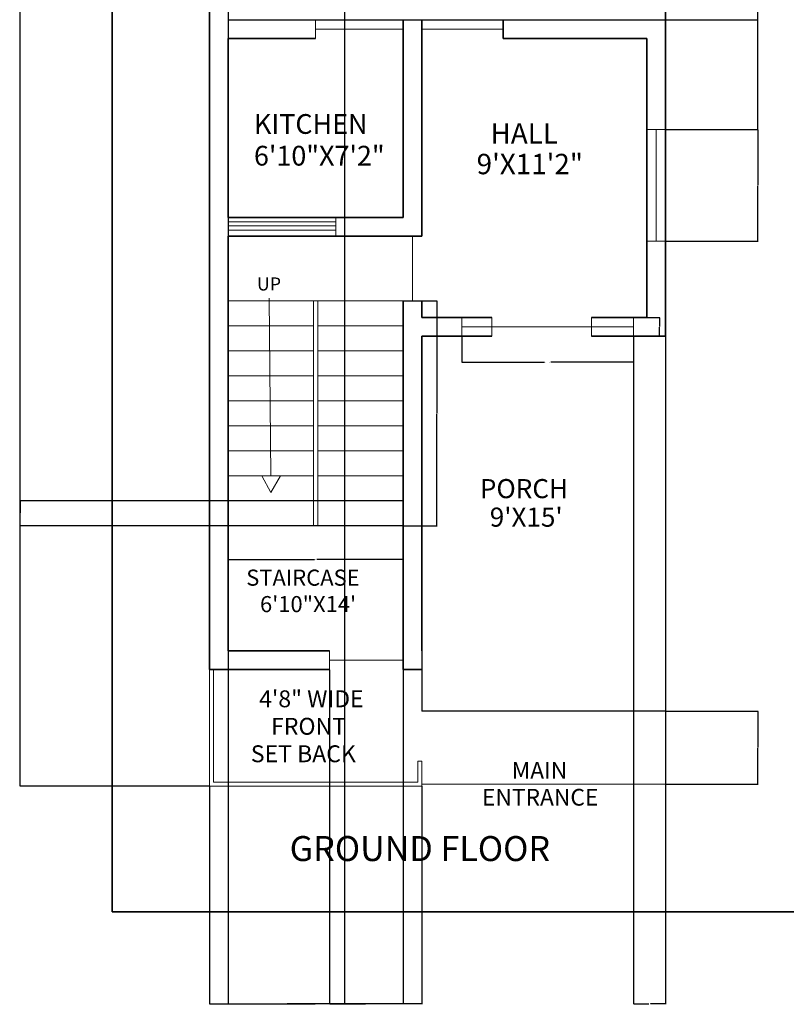
# Model space of a CAD drawing. Units: feet. Extents: x 2100 to 2836, y 2433 to 3396.
# Tile 1 of 12: x 2100 to 2468, y 2433 to 2906. Entities that reach past the tile are written whole.
import ezdxf

# ---------------------------------------------------------------- set-up
doc = ezdxf.new("R2010")
doc.units = ezdxf.units.FT
for name, color, linetype, lineweight in [('A-ANNO-DIMS', 2, 'Continuous', 18), ('A-ANNO-SYMB', 2, 'Continuous', 13), ('A-ANNO-TEXT', 7, 'Continuous', 18), ('A-ANNO-TITL', 7, 'Continuous', 25), ('A-ANNO-TTLB', 7, 'Continuous', 35), ('A-AREA-IDEN', 7, 'Continuous', 18), ('A-DOOR', 3, 'Continuous', 18), ('A-FLOR-EDGE', 7, 'Continuous', 25), ('A-FLOR-STRS', 2, 'Continuous', 20), ('A-GLAZ', 4, 'Continuous', 18), ('A-WALL', 7, 'Continuous', 35), ('C-PROP', 8, 'Continuous', 18)]:
    doc.layers.add(name, color=color, linetype=linetype, lineweight=lineweight)
doc.styles.get("Standard").update_dxf_attribs({"font": 'arial.ttf'})
doc.dimstyles.get("Standard").update_dxf_attribs({"dimtxt": 0.18, "dimasz": 0.18, "dimexe": 0.18, "dimexo": 0.0625, "dimgap": 0.09, "dimtad": 0, "dimtih": 1, "dimtoh": 1, "dimdec": 4, "dimzin": 0, "dimdsep": 46, "dimtxsty": 'Standard', "dimcen": 0.09, "dimadec": 0, "dimazin": 0, "dimtfac": 1, "dimtdec": 4, "dimtofl": 0, "dimtmove": 0, "dimatfit": 3, "dimfxl": 1, "dimtolj": 1, "dimtzin": 0, "dimarcsym": 0})

# ---------------------------------------------------------------- blocks, each defined once
blk = doc.blocks.new('STAIR-RETURN-FLIGHT')
for p, q in [((84, 108), (0, 108)), ((41, 108), (41, 0)), ((43, 108), (43, 0)), ((41, 96), (0, 96)), ((84, 96), (43, 96)), ((41, 84), (0, 84)), ((84, 84), (43, 84)), ((41, 72), (0, 72)), ((84, 72), (43, 72)), ((41, 60), (0, 60)), ((84, 60), (43, 60)), ((41, 48), (0, 48)), ((84, 48), (43, 48)), ((41, 36), (0, 36)), ((84, 36), (43, 36)), ((41, 24), (0, 24)), ((84, 24), (43, 24)), ((84, 12), (0, 12)), ((84, 0), (0, 0))]:
    blk.add_line(p, q)
blk = doc.blocks.new('STAIR-DIRECTION')
for p, q in [((3.63, 93.38), (4.37, 8)), ((4.44, 0), (0, 8)), ((4.44, 0), (8.95, 8))]:
    blk.add_line(p, q)
blk = doc.blocks.new('WIN-KITCHEN')
for p, q in [((0, 9), (0, 0)), ((51.75, 7), (0, 7)), ((51.75, 5), (0, 5)), ((51.75, 9), (51.75, 0)), ((51.75, 3), (0, 3))]:
    blk.add_line(p, q)
blk = doc.blocks.new('DOOR-STAIR-HALL')
for p, q in [((4.5, 0), (4.5, 31.05)), ((9, 0), (0, 0))]:
    blk.add_line(p, q)
blk = doc.blocks.new('DOOR-PASSAGE')
for p, q in [((42, 0), (42, 9)), ((42, 4.5), (0, 4.5))]:
    blk.add_line(p, q)
blk = doc.blocks.new('DOOR-SLIDING-ENTRY')
for p, q in [((0, 9), (0, 0)), ((14.54, 9), (14.54, 0)), ((62.31, 9), (62.31, 0)), ((82.55, 9), (82.55, 0)), ((0, 4.5), (82.55, 4.5))]:
    blk.add_line(p, q)
blk = doc.blocks.new('*D18')
at = {"layer": 'A-ANNO-DIMS', "color": 0, "lineweight": -2, "transparency": 16777216}
for p, q in [((2283.75, 2770.76), (2300.07, 2770.76)), ((2299.89, 2770.58), (2299.89, 2716.94)), ((2299.89, 2662.94), (2299.89, 2716.57)), ((2283.75, 2662.76), (2300.07, 2662.76))]:
    blk.add_line(p, q, dxfattribs=at)
at = {"layer": 'A-ANNO-DIMS', "color": 0, "transparency": 16777216}
for points in [[(2299.86, 2770.58), (2299.92, 2770.58), (2299.89, 2770.76)], [(2299.86, 2662.94), (2299.92, 2662.94), (2299.89, 2662.76)]]:
    blk.add_solid(points, dxfattribs=at)
at = {"layer": 'Defpoints', "color": 0, "transparency": 16777216}
for p in [(2283.69, 2770.76), (2299.89, 2770.76), (2283.69, 2662.76)]:
    blk.add_point(p, dxfattribs=at)
at = {"layer": 'A-ANNO-DIMS', "color": 0, "transparency": 16777216, "insert": (2299.89, 2716.76), "char_height": 0.18, "attachment_point": 5}
blk.add_mtext('\\A1;RETURN FLIGHT 108 TYP.', dxfattribs=at)
blk = doc.blocks.new('*D19')
at = {"layer": 'A-ANNO-DIMS', "color": 0, "lineweight": -2, "transparency": 16777216}
for p, q in [((2199.69, 2662.69), (2199.69, 2646.38)), ((2283.69, 2662.69), (2283.69, 2646.38)), ((2199.87, 2646.56), (2241.16, 2646.56)), ((2283.51, 2646.56), (2242.21, 2646.56))]:
    blk.add_line(p, q, dxfattribs=at)
at = {"layer": 'A-ANNO-DIMS', "color": 0, "transparency": 16777216}
for points in [[(2199.87, 2646.59), (2199.87, 2646.53), (2199.69, 2646.56)], [(2283.51, 2646.59), (2283.51, 2646.53), (2283.69, 2646.56)]]:
    blk.add_solid(points, dxfattribs=at)
at = {"layer": 'Defpoints', "color": 0, "transparency": 16777216}
for p in [(2199.69, 2662.76), (2283.69, 2662.76), (2283.69, 2646.56)]:
    blk.add_point(p, dxfattribs=at)
at = {"layer": 'A-ANNO-DIMS', "color": 0, "transparency": 16777216, "insert": (2241.69, 2646.56), "char_height": 0.18, "attachment_point": 5}
blk.add_mtext('\\A1;84 TYP.', dxfattribs=at)
blk = doc.blocks.new('*D38')
at = {"layer": 'A-ANNO-DIMS', "color": 0, "lineweight": -2, "transparency": 16777216}
for p, q in [((2311.81, 2753.74), (2311.81, 2741.24)), ((2394.36, 2753.74), (2394.36, 2741.24)), ((2311.99, 2741.42), (2351.56, 2741.42)), ((2394.18, 2741.42), (2354.61, 2741.42))]:
    blk.add_line(p, q, dxfattribs=at)
at = {"layer": 'A-ANNO-DIMS', "color": 0, "transparency": 16777216}
for points in [[(2311.99, 2741.45), (2311.99, 2741.39), (2311.81, 2741.42)], [(2394.18, 2741.45), (2394.18, 2741.39), (2394.36, 2741.42)]]:
    blk.add_solid(points, dxfattribs=at)
at = {"layer": 'Defpoints', "color": 0, "transparency": 16777216}
for p in [(2311.81, 2753.8), (2394.36, 2753.8), (2394.36, 2741.42)]:
    blk.add_point(p, dxfattribs=at)
at = {"layer": 'A-ANNO-DIMS', "color": 0, "transparency": 16777216, "insert": (2353.08, 2741.42), "char_height": 0.18, "attachment_point": 5}
blk.add_mtext('\\A1;SLIDING ENTRY 83 TYP.', dxfattribs=at)
blk = doc.blocks.new('*D39')
at = {"layer": 'A-ANNO-DIMS', "color": 0, "lineweight": -2, "transparency": 16777216}
for p, q in [((2394.42, 2762.8), (2406.92, 2762.8)), ((2406.74, 2762.62), (2406.74, 2758.48)), ((2406.74, 2753.98), (2406.74, 2758.12)), ((2394.42, 2753.8), (2406.92, 2753.8))]:
    blk.add_line(p, q, dxfattribs=at)
at = {"layer": 'A-ANNO-DIMS', "color": 0, "transparency": 16777216}
for points in [[(2406.71, 2762.62), (2406.77, 2762.62), (2406.74, 2762.8)], [(2406.71, 2753.98), (2406.77, 2753.98), (2406.74, 2753.8)]]:
    blk.add_solid(points, dxfattribs=at)
at = {"layer": 'Defpoints', "color": 0, "transparency": 16777216}
for p in [(2394.36, 2762.8), (2406.74, 2762.8), (2394.36, 2753.8)]:
    blk.add_point(p, dxfattribs=at)
at = {"layer": 'A-ANNO-DIMS', "color": 0, "transparency": 16777216, "insert": (2406.74, 2758.3), "char_height": 0.18, "attachment_point": 5}
blk.add_mtext('\\A1;9 TYP.', dxfattribs=at)
blk = doc.blocks.new('*D41')
at = {"layer": 'A-ANNO-DIMS', "color": 0, "lineweight": -2, "transparency": 16777216}
for p, q in [((2190.62, 3321.8), (2099.65, 3321.8)), ((2099.83, 3321.62), (2099.83, 2929.96)), ((2099.83, 2537.94), (2099.83, 2929.6)), ((2190.62, 2537.76), (2099.65, 2537.76))]:
    blk.add_line(p, q, dxfattribs=at)
at = {"layer": 'A-ANNO-DIMS', "color": 0, "transparency": 16777216}
for points in [[(2099.8, 3321.62), (2099.86, 3321.62), (2099.83, 3321.8)], [(2099.8, 2537.94), (2099.86, 2537.94), (2099.83, 2537.76)]]:
    blk.add_solid(points, dxfattribs=at)
at = {"layer": 'Defpoints', "color": 0, "transparency": 16777216}
for p in [(2099.83, 3321.8), (2190.69, 3321.8), (2190.69, 2537.76)]:
    blk.add_point(p, dxfattribs=at)
at = {"layer": 'A-ANNO-DIMS', "color": 0, "transparency": 16777216, "insert": (2099.83, 2929.78), "char_height": 0.18, "attachment_point": 5}
blk.add_mtext('\\A1;784', dxfattribs=at)
blk = doc.blocks.new('*D44')
at = {"layer": 'A-ANNO-DIMS', "color": 0, "lineweight": -2, "transparency": 16777216}
for p, q in [((2199.69, 3312.74), (2199.69, 2433.01)), ((2255.63, 3312.74), (2255.63, 2433.01)), ((2199.87, 2433.19), (2227.26, 2433.19)), ((2255.45, 2433.19), (2228.05, 2433.19))]:
    blk.add_line(p, q, dxfattribs=at)
at = {"layer": 'A-ANNO-DIMS', "color": 0, "transparency": 16777216}
for points in [[(2199.87, 2433.22), (2199.87, 2433.16), (2199.69, 2433.19)], [(2255.45, 2433.22), (2255.45, 2433.16), (2255.63, 2433.19)]]:
    blk.add_solid(points, dxfattribs=at)
at = {"layer": 'Defpoints', "color": 0, "transparency": 16777216}
for p in [(2199.69, 3312.8), (2255.63, 3312.8), (2255.63, 2433.19)]:
    blk.add_point(p, dxfattribs=at)
at = {"layer": 'A-ANNO-DIMS', "color": 0, "transparency": 16777216, "insert": (2227.66, 2433.19), "char_height": 0.18, "attachment_point": 5}
blk.add_mtext('\\A1;55.94', dxfattribs=at)
blk = doc.blocks.new('*D50')
at = {"layer": 'A-ANNO-DIMS', "color": 0, "lineweight": -2, "transparency": 16777216}
for p, q in [((2409.75, 3084.54), (2454.12, 3084.54)), ((2453.94, 3084.36), (2453.94, 2968.97)), ((2453.94, 2853.21), (2453.94, 2968.6)), ((2409.75, 2853.03), (2454.12, 2853.03))]:
    blk.add_line(p, q, dxfattribs=at)
at = {"layer": 'A-ANNO-DIMS', "color": 0, "transparency": 16777216}
for points in [[(2453.91, 3084.36), (2453.97, 3084.36), (2453.94, 3084.54)], [(2453.91, 2853.21), (2453.97, 2853.21), (2453.94, 2853.03)]]:
    blk.add_solid(points, dxfattribs=at)
at = {"layer": 'Defpoints', "color": 0, "transparency": 16777216}
for p in [(2409.69, 3084.54), (2409.69, 2853.03), (2453.94, 2853.03)]:
    blk.add_point(p, dxfattribs=at)
at = {"layer": 'A-ANNO-DIMS', "color": 0, "transparency": 16777216, "insert": (2453.94, 2968.78), "char_height": 0.18, "attachment_point": 5}
blk.add_mtext('\\A1;231.5', dxfattribs=at)
blk = doc.blocks.new('*D51')
at = {"layer": 'A-ANNO-DIMS', "color": 0, "lineweight": -2, "transparency": 16777216}
for p, q in [((2409.75, 2853.03), (2454.12, 2853.03)), ((2453.94, 2852.85), (2453.94, 2826.4)), ((2453.94, 2799.59), (2453.94, 2826.03)), ((2409.75, 2799.41), (2454.12, 2799.41))]:
    blk.add_line(p, q, dxfattribs=at)
at = {"layer": 'A-ANNO-DIMS', "color": 0, "transparency": 16777216}
for points in [[(2453.91, 2852.85), (2453.97, 2852.85), (2453.94, 2853.03)], [(2453.91, 2799.59), (2453.97, 2799.59), (2453.94, 2799.41)]]:
    blk.add_solid(points, dxfattribs=at)
at = {"layer": 'Defpoints', "color": 0, "transparency": 16777216}
for p in [(2409.69, 2853.03), (2409.69, 2799.41), (2453.94, 2799.41)]:
    blk.add_point(p, dxfattribs=at)
at = {"layer": 'A-ANNO-DIMS', "color": 0, "transparency": 16777216, "insert": (2453.94, 2826.22), "char_height": 0.18, "attachment_point": 5}
blk.add_mtext('\\A1;53.62', dxfattribs=at)
blk = doc.blocks.new('*D52')
at = {"layer": 'A-ANNO-DIMS', "color": 0, "lineweight": -2, "transparency": 16777216}
for p, q in [((2199.75, 2970.11), (2454.12, 2970.11)), ((2453.94, 2969.93), (2453.94, 2938.14)), ((2453.94, 2905.98), (2453.94, 2937.78)), ((2199.75, 2905.8), (2454.12, 2905.8))]:
    blk.add_line(p, q, dxfattribs=at)
at = {"layer": 'A-ANNO-DIMS', "color": 0, "transparency": 16777216}
for points in [[(2453.91, 2969.93), (2453.97, 2969.93), (2453.94, 2970.11)], [(2453.91, 2905.98), (2453.97, 2905.98), (2453.94, 2905.8)]]:
    blk.add_solid(points, dxfattribs=at)
at = {"layer": 'Defpoints', "color": 0, "transparency": 16777216}
for p in [(2199.69, 2970.11), (2453.94, 2970.11), (2199.69, 2905.8)]:
    blk.add_point(p, dxfattribs=at)
at = {"layer": 'A-ANNO-DIMS', "color": 0, "transparency": 16777216, "insert": (2453.94, 2937.96), "char_height": 0.18, "attachment_point": 5}
blk.add_mtext('\\A1;64.31', dxfattribs=at)
blk = doc.blocks.new('*D54')
at = {"layer": 'A-ANNO-DIMS', "color": 0, "lineweight": -2, "transparency": 16777216}
for p, q in [((2409.75, 2573.8), (2454.12, 2573.8)), ((2453.94, 2573.62), (2453.94, 2556.46)), ((2453.94, 2538.94), (2453.94, 2556.1)), ((2409.75, 2538.76), (2454.12, 2538.76))]:
    blk.add_line(p, q, dxfattribs=at)
at = {"layer": 'A-ANNO-DIMS', "color": 0, "transparency": 16777216}
for points in [[(2453.91, 2573.62), (2453.97, 2573.62), (2453.94, 2573.8)], [(2453.91, 2538.94), (2453.97, 2538.94), (2453.94, 2538.76)]]:
    blk.add_solid(points, dxfattribs=at)
at = {"layer": 'Defpoints', "color": 0, "transparency": 16777216}
for p in [(2409.69, 2573.8), (2453.94, 2573.8), (2409.69, 2538.76)]:
    blk.add_point(p, dxfattribs=at)
at = {"layer": 'A-ANNO-DIMS', "color": 0, "transparency": 16777216, "insert": (2453.94, 2556.28), "char_height": 0.18, "attachment_point": 5}
blk.add_mtext('\\A1;35.05', dxfattribs=at)
blk = doc.blocks.new('*D55')
at = {"layer": 'A-ANNO-DIMS', "color": 0, "lineweight": -2, "transparency": 16777216}
for p, q in [((2283.62, 2674.76), (2099.65, 2674.76)), ((2099.83, 2674.58), (2099.83, 2668.94)), ((2099.83, 2662.94), (2099.83, 2668.57)), ((2283.62, 2662.76), (2099.65, 2662.76))]:
    blk.add_line(p, q, dxfattribs=at)
at = {"layer": 'A-ANNO-DIMS', "color": 0, "transparency": 16777216}
for points in [[(2099.8, 2674.58), (2099.86, 2674.58), (2099.83, 2674.76)], [(2099.8, 2662.94), (2099.86, 2662.94), (2099.83, 2662.76)]]:
    blk.add_solid(points, dxfattribs=at)
at = {"layer": 'Defpoints', "color": 0, "transparency": 16777216}
for p in [(2099.83, 2674.76), (2283.69, 2674.76), (2283.69, 2662.76)]:
    blk.add_point(p, dxfattribs=at)
at = {"layer": 'A-ANNO-DIMS', "color": 0, "transparency": 16777216, "insert": (2099.83, 2668.76), "char_height": 0.18, "attachment_point": 5}
blk.add_mtext('\\A1;12', dxfattribs=at)
blk = doc.blocks.new('*D61')
at = {"layer": 'A-ANNO-DIMS', "color": 0, "lineweight": -2, "transparency": 16777216}
for p, q in [((2248.36, 2593.69), (2248.36, 2433.01)), ((2283.69, 2593.69), (2283.69, 2433.01)), ((2248.54, 2433.19), (2265.63, 2433.19)), ((2283.51, 2433.19), (2266.42, 2433.19))]:
    blk.add_line(p, q, dxfattribs=at)
at = {"layer": 'A-ANNO-DIMS', "color": 0, "transparency": 16777216}
for points in [[(2248.54, 2433.22), (2248.54, 2433.16), (2248.36, 2433.19)], [(2283.51, 2433.22), (2283.51, 2433.16), (2283.69, 2433.19)]]:
    blk.add_solid(points, dxfattribs=at)
at = {"layer": 'Defpoints', "color": 0, "transparency": 16777216}
for p in [(2248.36, 2593.76), (2283.69, 2593.76), (2283.69, 2433.19)]:
    blk.add_point(p, dxfattribs=at)
at = {"layer": 'A-ANNO-DIMS', "color": 0, "transparency": 16777216, "insert": (2266.02, 2433.19), "char_height": 0.18, "attachment_point": 5}
blk.add_mtext('\\A1;35.32', dxfattribs=at)
blk = doc.blocks.new('*D64')
at = {"layer": 'A-ANNO-DIMS', "color": 0, "lineweight": -2, "transparency": 16777216}
for p, q in [((2394.36, 2753.74), (2394.36, 2433.01)), ((2409.69, 2753.74), (2409.69, 2433.01)), ((2394.54, 2433.19), (2401.64, 2433.19)), ((2409.51, 2433.19), (2402.41, 2433.19))]:
    blk.add_line(p, q, dxfattribs=at)
at = {"layer": 'A-ANNO-DIMS', "color": 0, "transparency": 16777216}
for points in [[(2394.54, 2433.22), (2394.54, 2433.16), (2394.36, 2433.19)], [(2409.51, 2433.22), (2409.51, 2433.16), (2409.69, 2433.19)]]:
    blk.add_solid(points, dxfattribs=at)
at = {"layer": 'Defpoints', "color": 0, "transparency": 16777216}
for p in [(2394.36, 2753.8), (2409.69, 2753.8), (2409.69, 2433.19)]:
    blk.add_point(p, dxfattribs=at)
at = {"layer": 'A-ANNO-DIMS', "color": 0, "transparency": 16777216, "insert": (2402.02, 2433.19), "char_height": 0.18, "attachment_point": 5}
blk.add_mtext('\\A1;15.33', dxfattribs=at)
blk = doc.blocks.new('*D67')
at = {"layer": 'A-ANNO-DIMS', "color": 0, "lineweight": -2, "transparency": 16777216}
for p, q in [((2190.69, 2537.69), (2190.69, 2433.01)), ((2292.69, 2537.69), (2292.69, 2433.01)), ((2190.87, 2433.19), (2241.41, 2433.19)), ((2292.51, 2433.19), (2241.97, 2433.19))]:
    blk.add_line(p, q, dxfattribs=at)
at = {"layer": 'A-ANNO-DIMS', "color": 0, "transparency": 16777216}
for points in [[(2190.87, 2433.22), (2190.87, 2433.16), (2190.69, 2433.19)], [(2292.51, 2433.22), (2292.51, 2433.16), (2292.69, 2433.19)]]:
    blk.add_solid(points, dxfattribs=at)
at = {"layer": 'Defpoints', "color": 0, "transparency": 16777216}
for p in [(2190.69, 2537.76), (2292.69, 2537.76), (2292.69, 2433.19)]:
    blk.add_point(p, dxfattribs=at)
at = {"layer": 'A-ANNO-DIMS', "color": 0, "transparency": 16777216, "insert": (2241.69, 2433.19), "char_height": 0.18, "attachment_point": 5}
blk.add_mtext('\\A1;102', dxfattribs=at)

msp = doc.modelspace()

# ---------------------------------------------------------------- linework, layer by layer
at = {"layer": 'A-ANNO-TTLB'}
msp.add_lwpolyline([(2144.0848, 3351.6245), (2791.0561, 3351.6245), (2791.0561, 2477.4373), (2144.0848, 2477.4373)], close=True, dxfattribs=at)
at = {"layer": 'A-DOOR'}
for p, q in [((2292.6857, 2901.3031), (2331.6857, 2901.3031)), ((2248.364, 2602.755), (2248.364, 2593.755)), ((2248.364, 2598.255), (2283.6857, 2598.255))]:
    msp.add_line(p, q, dxfattribs=at)
at = {"layer": 'A-FLOR-EDGE'}
for p in [(2292.6857, 2602.755), (2409.6857, 2573.8031)]:
    msp.add_line(p, (2292.6857, 2573.8031), dxfattribs=at)
at = {"layer": 'A-GLAZ'}
for p, q in [((2400.6857, 2853.0255), (2409.6857, 2853.0255)), ((2405.1857, 2853.0255), (2405.1857, 2799.4059)), ((2400.6857, 2799.4059), (2409.6857, 2799.4059))]:
    msp.add_line(p, q, dxfattribs=at)
at = {"layer": 'A-WALL'}
for p, q in [((2190.6857, 2593.755), (2190.6857, 3321.8031)), ((2409.6857, 2987.2733), (2409.6857, 2891.1053)), ((2283.6857, 2810.8031), (2283.6857, 2905.8031)), ((2292.6857, 2801.8031), (2292.6857, 2905.8031)), ((2331.6857, 2905.8031), (2331.6857, 2896.8031)), ((2241.6857, 2896.8031), (2199.6857, 2896.8031)), ((2199.6857, 2810.8031), (2199.6857, 2896.8031)), ((2331.6857, 2896.8031), (2400.6857, 2896.8031)), ((2400.6857, 2896.8031), (2400.6857, 2762.8031)), ((2409.6857, 2896.8031), (2409.6857, 2753.8031)), ((2283.6857, 2810.8031), (2199.6857, 2810.8031)), ((2199.6857, 2602.755), (2199.6857, 2801.8031)), ((2292.6857, 2801.8031), (2199.6857, 2801.8031)), ((2283.6857, 2753.8031), (2283.6857, 2770.755)), ((2283.6857, 2770.755), (2283.6857, 2602.755)), ((2292.6857, 2762.8031), (2292.6857, 2770.755)), ((2292.6857, 2770.755), (2292.6857, 2762.8031)), ((2326.3537, 2762.8031), (2292.6857, 2762.8031)), ((2400.6857, 2762.8031), (2374.1147, 2762.8031)), ((2292.6857, 2753.8031), (2292.6857, 2602.755)), ((2326.3537, 2753.8031), (2292.6857, 2753.8031)), ((2409.6857, 2753.8031), (2374.1147, 2753.8031)), ((2248.364, 2602.755), (2199.6857, 2602.755)), ((2283.6857, 2602.755), (2283.6857, 2593.755)), ((2248.364, 2593.755), (2190.6857, 2593.755)), ((2292.6857, 2593.755), (2283.6857, 2593.755))]:
    msp.add_line(p, q, dxfattribs=at)
at = {"layer": 'C-PROP'}
for p, q in [((2409.6857, 2753.8031), (2409.6857, 2538.755)), ((2190.6857, 2593.755), (2190.6857, 2537.755)), ((2192.6857, 2593.755), (2192.6857, 2539.755)), ((2290.6857, 2539.755), (2290.6857, 2549.7146)), ((2292.6857, 2549.7146), (2290.6857, 2549.7146)), ((2292.6857, 2539.755), (2292.6857, 2549.7146)), ((2192.6857, 2539.755), (2290.6857, 2539.755)), ((2292.6857, 2539.755), (2292.6857, 2537.755)), ((2190.6857, 2537.755), (2292.6857, 2537.755)), ((2292.6857, 2538.755), (2409.6857, 2538.755))]:
    msp.add_line(p, q, dxfattribs=at)

# ---------------------------------------------------------------- block references
at = {"layer": 'A-ANNO-SYMB'}
msp.add_blockref('STAIR-DIRECTION', (2215.817, 2678.7553), dxfattribs=at)
at = {"layer": 'A-DOOR', "rotation": 180}
msp.add_blockref('DOOR-PASSAGE', (2283.6857, 2905.8031), dxfattribs=at)
at = {"layer": 'A-DOOR'}
for name, p in [('DOOR-STAIR-HALL', (2283.6857, 2770.755)), ('DOOR-SLIDING-ENTRY', (2311.8093, 2753.8031))]:
    msp.add_blockref(name, p, dxfattribs=at)
at = {"layer": 'A-FLOR-STRS'}
msp.add_blockref('STAIR-RETURN-FLIGHT', (2199.6857, 2662.755), dxfattribs=at)
at = {"layer": 'A-GLAZ'}
msp.add_blockref('WIN-KITCHEN', (2199.6857, 2801.8031), dxfattribs=at)

# ---------------------------------------------------------------- texts
at = {"layer": 'A-ANNO-TEXT'}
for s, height, p in [('UP', 6.26655, (2213.5142, 2775.7836)), ('MAIN', 8.02214, (2335.8327, 2541.3138)), ('ENTRANCE', 8.02214, (2321.5652, 2528.4245))]:
    msp.add_text(s, height=height, dxfattribs=at).set_placement(p)
at = {"layer": 'A-ANNO-TITL'}
msp.add_text('GROUND FLOOR', height=12, dxfattribs=at).set_placement((2229.2448, 2501.7888))
at = {"layer": 'A-AREA-IDEN'}
for s, height, p in [('KITCHEN', 9.48042, (2212.086, 2850.9877)), ('HALL', 9.79205, (2325.6794, 2846.3015)), ('6\'10"X7\'2"', 9.48042, (2212.086, 2835.7582)), ('9\'X11\'2"', 9.79205, (2318.9928, 2831.5994)), ('PORCH', 9.18056, (2320.5563, 2676.0395)), ("9'X15'", 9.18056, (2325.3007, 2662.3452)), ('STAIRCASE', 7.73004, (2208.3758, 2634.0152)), ('6\'10"X14\'', 7.73004, (2214.9821, 2621.3093)), ('4\'8" WIDE', 8.11145, (2214.5658, 2575.6461)), ('FRONT ', 8.11145, (2220.3218, 2562.4514)), ('SET BACK', 8.11145, (2210.5752, 2549.2525))]:
    msp.add_text(s, height=height, dxfattribs=at).set_placement(p)

# ---------------------------------------------------------------- dimensions: what is measured, and where the dimension line sits
at = {"layer": 'A-ANNO-DIMS'}
for base, p1, p2, override, picture, middle in [((2099.8348, 3321.8031), (2190.6857, 2537.755), (2190.6857, 3321.8031), {"dimdec": 0, "dimlfac": 1, "dimrnd": 0, "dimzin": 0, "dimdsep": 46, "dimlunit": 2}, '*D41', (2099.8348, 2929.7791)), ((2453.9357, 2853.0255), (2409.6857, 3084.5411), (2409.6857, 2853.0255), {"dimdec": 1, "dimlfac": 1, "dimrnd": 0, "dimzin": 0, "dimdsep": 46, "dimlunit": 2}, '*D50', (2453.9357, 2968.7833)), ((2453.9357, 2970.1128), (2199.6857, 2905.8031), (2199.6857, 2970.1128), {"dimdec": 2, "dimlfac": 1, "dimrnd": 0, "dimzin": 0, "dimdsep": 46, "dimlunit": 2}, '*D52', (2453.9357, 2937.9579)), ((2453.9357, 2799.4059), (2409.6857, 2853.0255), (2409.6857, 2799.4059), {"dimdec": 2, "dimlfac": 1, "dimrnd": 0, "dimzin": 0, "dimdsep": 46, "dimlunit": 2}, '*D51', (2453.9357, 2826.2157)), ((2099.8348, 2674.755), (2283.6857, 2662.755), (2283.6857, 2674.755), {"dimdec": 0, "dimlfac": 1, "dimrnd": 0, "dimzin": 0, "dimdsep": 46, "dimlunit": 2}, '*D55', (2099.8348, 2668.755)), ((2453.9357, 2573.8031), (2409.6857, 2538.755), (2409.6857, 2573.8031), {"dimdec": 2, "dimlfac": 1, "dimrnd": 0, "dimzin": 0, "dimdsep": 46, "dimlunit": 2}, '*D54', (2453.9357, 2556.2791))]:
    dim = msp.add_linear_dim(base=base, p1=p1, p2=p2, angle=90, dimstyle='Standard', override=override, dxfattribs=at)
    dim.commit()
    dim.dimension.update_dxf_attribs({"geometry": picture, "text_midpoint": middle})
for base, p1, p2, override, picture, middle in [((2255.625, 2433.1873), (2199.6857, 3312.8031), (2255.625, 3312.8031), {"dimdec": 2, "dimlfac": 1, "dimrnd": 0, "dimzin": 0, "dimdsep": 46, "dimlunit": 2}, '*D44', (2227.6554, 2433.1873)), ((2409.6857, 2433.1873), (2394.3555, 2753.8031), (2409.6857, 2753.8031), {"dimdec": 2, "dimlfac": 1, "dimrnd": 0, "dimzin": 0, "dimdsep": 46, "dimlunit": 2}, '*D64', (2402.0206, 2433.1873)), ((2283.6857, 2433.1873), (2248.364, 2593.755), (2283.6857, 2593.755), {"dimdec": 2, "dimlfac": 1, "dimrnd": 0, "dimzin": 0, "dimdsep": 46, "dimlunit": 2}, '*D61', (2266.0248, 2433.1873)), ((2292.6857, 2433.1873), (2190.6857, 2537.755), (2292.6857, 2537.755), {"dimdec": 0, "dimlfac": 1, "dimrnd": 0, "dimzin": 0, "dimdsep": 46, "dimlunit": 2}, '*D67', (2241.6857, 2433.1873))]:
    dim = msp.add_linear_dim(base=base, p1=p1, p2=p2, dimstyle='Standard', override=override, dxfattribs=at)
    dim.commit()
    dim.dimension.update_dxf_attribs({"geometry": picture, "text_midpoint": middle})
for base, p1, p2, text, picture, middle in [((2299.8857, 2770.755), (2283.6857, 2662.755), (2283.6857, 2770.755), 'RETURN FLIGHT <> TYP.', '*D18', (2299.8857, 2716.755)), ((2406.7374, 2762.8031), (2394.3555, 2753.8031), (2394.3555, 2762.8031), '<> TYP.', '*D39', (2406.7374, 2758.3031))]:
    dim = msp.add_linear_dim(base=base, p1=p1, p2=p2, angle=90, text=text, dimstyle='Standard', override={"dimdec": 0, "dimlfac": 1, "dimrnd": 0, "dimzin": 0, "dimdsep": 46, "dimlunit": 2}, dxfattribs=at)
    dim.commit()
    dim.dimension.update_dxf_attribs({"geometry": picture, "text_midpoint": middle})
for base, p1, p2, text, picture, middle in [((2394.3555, 2741.4211), (2311.8093, 2753.8031), (2394.3555, 2753.8031), 'SLIDING ENTRY <> TYP.', '*D38', (2353.0824, 2741.4211)), ((2283.6857, 2646.555), (2199.6857, 2662.755), (2283.6857, 2662.755), '<> TYP.', '*D19', (2241.6857, 2646.555))]:
    dim = msp.add_linear_dim(base=base, p1=p1, p2=p2, text=text, dimstyle='Standard', override={"dimdec": 0, "dimlfac": 1, "dimrnd": 0, "dimzin": 0, "dimdsep": 46, "dimlunit": 2}, dxfattribs=at)
    dim.commit()
    dim.dimension.update_dxf_attribs({"geometry": picture, "text_midpoint": middle})

doc.saveas('drawing.dxf')
